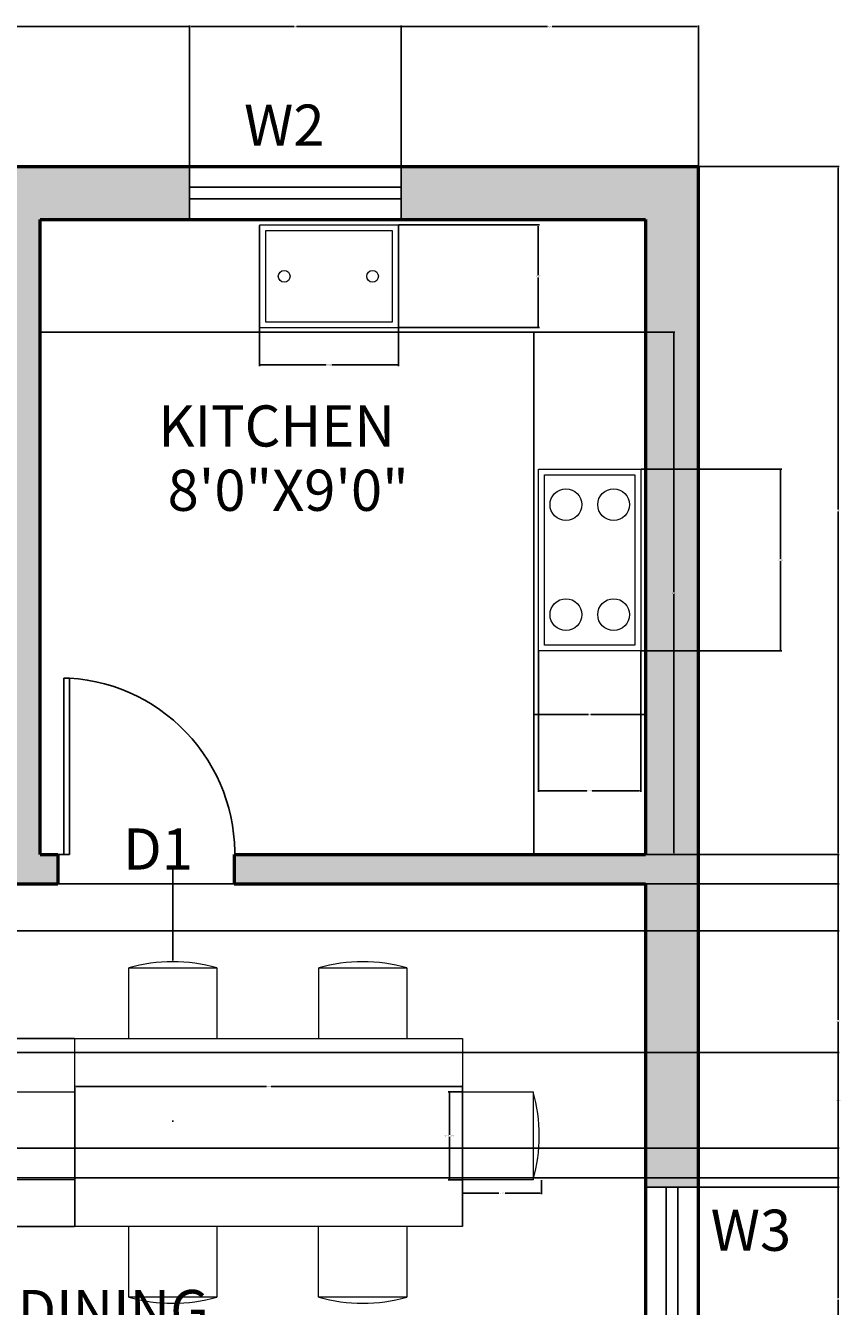
# Model space of a CAD drawing. Units: inches. Extents: x 2715 to 3027, y 1777 to 2287.
# Tile 4 of 4: x 2888 to 3027, y 2069 to 2287. Entities that reach past the tile are written whole.
import ezdxf

# ---------------------------------------------------------------- set-up
doc = ezdxf.new("R2010")
doc.units = ezdxf.units.IN
for name, color, linetype, lineweight in [('A-ANNO-DIMS', 2, 'Continuous', 18), ('A-ANNO-TEXT', 2, 'Continuous', 18), ('A-AREA-IDEN', 2, 'Continuous', 18), ('A-DOOR', 111, 'Continuous', 25), ('A-EQPM', 57, 'Continuous', 18), ('A-FLOR-CASE', 201, 'Continuous', 25), ('A-FLOR-FIXT', 201, 'Continuous', 18), ('A-FURN', 201, 'Continuous', 18), ('A-GLAZ', 40, 'Continuous', 25), ('A-WALL', 7, 'Continuous', 50), ('A-WALL-PATT', 252, 'Continuous', 13)]:
    doc.layers.add(name, color=color, linetype=linetype, lineweight=lineweight)
doc.styles.get("Standard").update_dxf_attribs({"font": 'arial.ttf'})
doc.dimstyles.get("Standard").update_dxf_attribs({"dimtxt": 0.18, "dimasz": 0.18, "dimexe": 0.18, "dimexo": 0.0625, "dimgap": 0.09, "dimtad": 0, "dimtih": 1, "dimtoh": 1, "dimdec": 4, "dimzin": 0, "dimdsep": 46, "dimtxsty": 'Standard', "dimcen": 0.09, "dimadec": 0, "dimazin": 0, "dimtfac": 1, "dimtdec": 4, "dimtofl": 0, "dimtmove": 0, "dimatfit": 3, "dimfxl": 1, "dimtolj": 1, "dimtzin": 0, "dimarcsym": 0})

# ---------------------------------------------------------------- blocks, each defined once
blk = doc.blocks.new('CHAIR-DINING')
for p, q in [((0, 0), (0, 12)), ((0, 12), (15, 12)), ((15, 12), (15, 0))]:
    blk.add_line(p, q)
blk.add_arc((7.5, -14.05), 27.1, 73.936, 106.064)
blk = doc.blocks.new('DOOR-SWING-30')
for p, q in [((29.11, 32.5), (28.11, 32.5)), ((28.11, 32.5), (28.11, 2.5)), ((29.11, 2.5), (29.11, 32.5)), ((28.11, 2.5), (29.11, 2.5)), ((30.11, 2.5), (29.11, 2.5))]:
    blk.add_line(p, q)
blk.add_arc((30, 2.56), 30, 93.6132, 184.8945)
blk = doc.blocks.new('*D11')
at = {"layer": 'A-ANNO-DIMS', "color": 0, "lineweight": -2, "transparency": 16777216}
for p, q in [((2962.73, 2105.97), (2960.36, 2105.97)), ((2960.54, 2105.79), (2960.54, 2098.66)), ((2960.54, 2091.15), (2960.54, 2098.29)), ((2962.73, 2090.97), (2960.36, 2090.97))]:
    blk.add_line(p, q, dxfattribs=at)
at = {"layer": 'A-ANNO-DIMS', "color": 0, "transparency": 16777216}
for points in [[(2960.51, 2105.79), (2960.57, 2105.79), (2960.54, 2105.97)], [(2960.51, 2091.15), (2960.57, 2091.15), (2960.54, 2090.97)]]:
    blk.add_solid(points, dxfattribs=at)
at = {"layer": 'Defpoints', "color": 0, "transparency": 16777216}
for p in [(2962.79, 2105.97), (2960.54, 2090.97), (2962.79, 2090.97)]:
    blk.add_point(p, dxfattribs=at)
at = {"layer": 'A-ANNO-DIMS', "color": 0, "transparency": 16777216, "insert": (2960.54, 2098.47), "char_height": 0.18, "attachment_point": 5}
blk.add_mtext('\\A1;CHAIR 15 TYP.', dxfattribs=at)
blk = doc.blocks.new('*D12')
at = {"layer": 'A-ANNO-DIMS', "color": 0, "lineweight": -2, "transparency": 16777216}
for p, q in [((2962.79, 2090.91), (2962.79, 2088.54)), ((2976.2, 2090.91), (2976.2, 2088.54)), ((2962.97, 2088.72), (2968.98, 2088.72)), ((2976.02, 2088.72), (2970.02, 2088.72))]:
    blk.add_line(p, q, dxfattribs=at)
at = {"layer": 'A-ANNO-DIMS', "color": 0, "transparency": 16777216}
for points in [[(2962.97, 2088.75), (2962.97, 2088.69), (2962.79, 2088.72)], [(2976.02, 2088.75), (2976.02, 2088.69), (2976.2, 2088.72)]]:
    blk.add_solid(points, dxfattribs=at)
at = {"layer": 'Defpoints', "color": 0, "transparency": 16777216}
for p in [(2962.79, 2090.97), (2976.2, 2090.97), (2976.2, 2088.72)]:
    blk.add_point(p, dxfattribs=at)
at = {"layer": 'A-ANNO-DIMS', "color": 0, "transparency": 16777216, "insert": (2969.5, 2088.72), "char_height": 0.18, "attachment_point": 5}
blk.add_mtext('\\A1;13 TYP.', dxfattribs=at)
blk = doc.blocks.new('*D30')
at = {"layer": 'A-ANNO-DIMS', "color": 0, "lineweight": -2, "transparency": 16777216}
for p, q in [((3002.98, 2089.72), (3026.9, 2089.72)), ((3026.72, 2089.54), (3026.72, 2070.9)), ((3026.72, 2051.9), (3026.72, 2070.54)), ((3002.98, 2051.72), (3026.9, 2051.72))]:
    blk.add_line(p, q, dxfattribs=at)
at = {"layer": 'A-ANNO-DIMS', "color": 0, "transparency": 16777216}
for points in [[(3026.69, 2089.54), (3026.75, 2089.54), (3026.72, 2089.72)], [(3026.69, 2051.9), (3026.75, 2051.9), (3026.72, 2051.72)]]:
    blk.add_solid(points, dxfattribs=at)
at = {"layer": 'Defpoints', "color": 0, "transparency": 16777216}
for p in [(3002.92, 2089.72), (3026.72, 2089.72), (3002.92, 2051.72)]:
    blk.add_point(p, dxfattribs=at)
at = {"layer": 'A-ANNO-DIMS', "color": 0, "transparency": 16777216, "insert": (3026.72, 2070.72), "char_height": 0.18, "attachment_point": 5}
blk.add_mtext('\\A1;38', dxfattribs=at)
blk = doc.blocks.new('*D31')
at = {"layer": 'A-ANNO-DIMS', "color": 0, "lineweight": -2, "transparency": 16777216}
for p, q in [((2993.98, 2146.34), (3026.9, 2146.34)), ((3026.72, 2146.16), (3026.72, 2118.21)), ((3026.72, 2089.9), (3026.72, 2117.85)), ((3002.98, 2089.72), (3026.9, 2089.72))]:
    blk.add_line(p, q, dxfattribs=at)
at = {"layer": 'A-ANNO-DIMS', "color": 0, "transparency": 16777216}
for points in [[(3026.69, 2146.16), (3026.75, 2146.16), (3026.72, 2146.34)], [(3026.69, 2089.9), (3026.75, 2089.9), (3026.72, 2089.72)]]:
    blk.add_solid(points, dxfattribs=at)
at = {"layer": 'Defpoints', "color": 0, "transparency": 16777216}
for p in [(2993.92, 2146.34), (3026.72, 2146.34), (3002.92, 2089.72)]:
    blk.add_point(p, dxfattribs=at)
at = {"layer": 'A-ANNO-DIMS', "color": 0, "transparency": 16777216, "insert": (3026.72, 2118.03), "char_height": 0.18, "attachment_point": 5}
blk.add_mtext('\\A1;56.62', dxfattribs=at)
blk = doc.blocks.new('*D32')
at = {"layer": 'A-ANNO-DIMS', "color": 0, "lineweight": -2, "transparency": 16777216}
for p, q in [((3002.98, 2263.34), (3026.9, 2263.34)), ((3026.72, 2263.16), (3026.72, 2205.02)), ((3026.72, 2146.52), (3026.72, 2204.66)), ((2993.98, 2146.34), (3026.9, 2146.34))]:
    blk.add_line(p, q, dxfattribs=at)
at = {"layer": 'A-ANNO-DIMS', "color": 0, "transparency": 16777216}
for points in [[(3026.69, 2263.16), (3026.75, 2263.16), (3026.72, 2263.34)], [(3026.69, 2146.52), (3026.75, 2146.52), (3026.72, 2146.34)]]:
    blk.add_solid(points, dxfattribs=at)
at = {"layer": 'Defpoints', "color": 0, "transparency": 16777216}
for p in [(3002.92, 2263.34), (3026.72, 2263.34), (2993.92, 2146.34)]:
    blk.add_point(p, dxfattribs=at)
at = {"layer": 'A-ANNO-DIMS', "color": 0, "transparency": 16777216, "insert": (3026.72, 2204.84), "char_height": 0.18, "attachment_point": 5}
blk.add_mtext('\\A1;117', dxfattribs=at)
blk = doc.blocks.new('*D35')
at = {"layer": 'A-ANNO-DIMS', "color": 0, "lineweight": -2, "transparency": 16777216}
for p, q in [((2823.27, 2263.4), (2823.27, 2287.33)), ((2823.45, 2287.15), (2869.41, 2287.15)), ((2916.16, 2287.15), (2870.19, 2287.15)), ((2916.34, 2263.4), (2916.34, 2287.33))]:
    blk.add_line(p, q, dxfattribs=at)
at = {"layer": 'A-ANNO-DIMS', "color": 0, "transparency": 16777216}
for points in [[(2823.45, 2287.18), (2823.45, 2287.12), (2823.27, 2287.15)], [(2916.16, 2287.18), (2916.16, 2287.12), (2916.34, 2287.15)]]:
    blk.add_solid(points, dxfattribs=at)
at = {"layer": 'Defpoints', "color": 0, "transparency": 16777216}
for p in [(2916.34, 2287.15), (2823.27, 2263.34), (2916.34, 2263.34)]:
    blk.add_point(p, dxfattribs=at)
at = {"layer": 'A-ANNO-DIMS', "color": 0, "transparency": 16777216, "insert": (2869.8, 2287.15), "char_height": 0.18, "attachment_point": 5}
blk.add_mtext('\\A1;93.07', dxfattribs=at)
blk = doc.blocks.new('*D36')
at = {"layer": 'A-ANNO-DIMS', "color": 0, "lineweight": -2, "transparency": 16777216}
for p, q in [((2916.34, 2263.4), (2916.34, 2287.33)), ((2916.52, 2287.15), (2934.12, 2287.15)), ((2952.16, 2287.15), (2934.55, 2287.15)), ((2952.34, 2263.4), (2952.34, 2287.33))]:
    blk.add_line(p, q, dxfattribs=at)
at = {"layer": 'A-ANNO-DIMS', "color": 0, "transparency": 16777216}
for points in [[(2916.52, 2287.18), (2916.52, 2287.12), (2916.34, 2287.15)], [(2952.16, 2287.18), (2952.16, 2287.12), (2952.34, 2287.15)]]:
    blk.add_solid(points, dxfattribs=at)
at = {"layer": 'Defpoints', "color": 0, "transparency": 16777216}
for p in [(2952.34, 2287.15), (2916.34, 2263.34), (2952.34, 2263.34)]:
    blk.add_point(p, dxfattribs=at)
at = {"layer": 'A-ANNO-DIMS', "color": 0, "transparency": 16777216, "insert": (2934.34, 2287.15), "char_height": 0.18, "attachment_point": 5}
blk.add_mtext('\\A1;36', dxfattribs=at)
blk = doc.blocks.new('*D37')
at = {"layer": 'A-ANNO-DIMS', "color": 0, "lineweight": -2, "transparency": 16777216}
for p, q in [((2952.34, 2263.4), (2952.34, 2287.33)), ((2952.52, 2287.15), (2977.23, 2287.15)), ((3002.74, 2287.15), (2978.02, 2287.15)), ((3002.92, 2263.4), (3002.92, 2287.33))]:
    blk.add_line(p, q, dxfattribs=at)
at = {"layer": 'A-ANNO-DIMS', "color": 0, "transparency": 16777216}
for points in [[(2952.52, 2287.18), (2952.52, 2287.12), (2952.34, 2287.15)], [(3002.74, 2287.18), (3002.74, 2287.12), (3002.92, 2287.15)]]:
    blk.add_solid(points, dxfattribs=at)
at = {"layer": 'Defpoints', "color": 0, "transparency": 16777216}
for p in [(3002.92, 2287.15), (2952.34, 2263.34), (3002.92, 2263.34)]:
    blk.add_point(p, dxfattribs=at)
at = {"layer": 'A-ANNO-DIMS', "color": 0, "transparency": 16777216, "insert": (2977.63, 2287.15), "char_height": 0.18, "attachment_point": 5}
blk.add_mtext('\\A1;50.58', dxfattribs=at)
blk = doc.blocks.new('*D41')
at = {"layer": 'A-ANNO-DIMS', "color": 0, "lineweight": -2, "transparency": 16777216}
for p, q in [((2747.98, 2112.64), (3026.9, 2112.64)), ((3026.72, 2112.46), (3026.72, 2104.67)), ((3026.72, 2096.52), (3026.72, 2104.31)), ((2747.98, 2096.34), (3026.9, 2096.34))]:
    blk.add_line(p, q, dxfattribs=at)
at = {"layer": 'A-ANNO-DIMS', "color": 0, "transparency": 16777216}
for points in [[(3026.69, 2112.46), (3026.75, 2112.46), (3026.72, 2112.64)], [(3026.69, 2096.52), (3026.75, 2096.52), (3026.72, 2096.34)]]:
    blk.add_solid(points, dxfattribs=at)
at = {"layer": 'Defpoints', "color": 0, "transparency": 16777216}
for p in [(2747.92, 2112.64), (3026.72, 2112.64), (2747.92, 2096.34)]:
    blk.add_point(p, dxfattribs=at)
at = {"layer": 'A-ANNO-DIMS', "color": 0, "transparency": 16777216, "insert": (3026.72, 2104.49), "char_height": 0.18, "attachment_point": 5}
blk.add_mtext('\\A1;16.297', dxfattribs=at)
blk = doc.blocks.new('*D42')
at = {"layer": 'A-ANNO-DIMS', "color": 0, "lineweight": -2, "transparency": 16777216}
for p, q in [((2831.98, 2141.34), (3026.9, 2141.34)), ((3026.72, 2141.16), (3026.72, 2137.52)), ((3026.72, 2133.52), (3026.72, 2137.16)), ((2831.98, 2133.34), (3026.9, 2133.34))]:
    blk.add_line(p, q, dxfattribs=at)
at = {"layer": 'A-ANNO-DIMS', "color": 0, "transparency": 16777216}
for points in [[(3026.69, 2141.16), (3026.75, 2141.16), (3026.72, 2141.34)], [(3026.69, 2133.52), (3026.75, 2133.52), (3026.72, 2133.34)]]:
    blk.add_solid(points, dxfattribs=at)
at = {"layer": 'Defpoints', "color": 0, "transparency": 16777216}
for p in [(2831.92, 2141.34), (3026.72, 2141.34), (2831.92, 2133.34)]:
    blk.add_point(p, dxfattribs=at)
at = {"layer": 'A-ANNO-DIMS', "color": 0, "transparency": 16777216, "insert": (3026.72, 2137.34), "char_height": 0.18, "attachment_point": 5}
blk.add_mtext('\\A1;8', dxfattribs=at)
blk = doc.blocks.new('*D43')
at = {"layer": 'A-ANNO-DIMS', "color": 0, "lineweight": -2, "transparency": 16777216}
for p, q in [((2747.98, 2096.34), (3026.9, 2096.34)), ((3026.72, 2096.16), (3026.72, 2094.02)), ((3026.72, 2091.52), (3026.72, 2093.66)), ((2747.98, 2091.34), (3026.9, 2091.34))]:
    blk.add_line(p, q, dxfattribs=at)
at = {"layer": 'A-ANNO-DIMS', "color": 0, "transparency": 16777216}
for points in [[(3026.69, 2096.16), (3026.75, 2096.16), (3026.72, 2096.34)], [(3026.69, 2091.52), (3026.75, 2091.52), (3026.72, 2091.34)]]:
    blk.add_solid(points, dxfattribs=at)
at = {"layer": 'Defpoints', "color": 0, "transparency": 16777216}
for p in [(2747.92, 2096.34), (3026.72, 2096.34), (2747.92, 2091.34)]:
    blk.add_point(p, dxfattribs=at)
at = {"layer": 'A-ANNO-DIMS', "color": 0, "transparency": 16777216, "insert": (3026.72, 2093.84), "char_height": 0.18, "attachment_point": 5}
blk.add_mtext('\\A1;5', dxfattribs=at)
blk = doc.blocks.new('*D51')
at = {"layer": 'A-ANNO-DIMS', "color": 0, "lineweight": -2, "transparency": 16777216}
for p, q in [((2896.82, 2083.1), (2896.82, 2107.02)), ((2962.79, 2083.1), (2962.79, 2107.02)), ((2897, 2106.84), (2929.41, 2106.84)), ((2962.61, 2106.84), (2930.2, 2106.84))]:
    blk.add_line(p, q, dxfattribs=at)
at = {"layer": 'A-ANNO-DIMS', "color": 0, "transparency": 16777216}
for points in [[(2897, 2106.87), (2897, 2106.81), (2896.82, 2106.84)], [(2962.61, 2106.87), (2962.61, 2106.81), (2962.79, 2106.84)]]:
    blk.add_solid(points, dxfattribs=at)
at = {"layer": 'Defpoints', "color": 0, "transparency": 16777216}
for p in [(2962.79, 2106.84), (2896.82, 2083.04), (2962.79, 2083.04)]:
    blk.add_point(p, dxfattribs=at)
at = {"layer": 'A-ANNO-DIMS', "color": 0, "transparency": 16777216, "insert": (2929.81, 2106.84), "char_height": 0.18, "attachment_point": 5}
blk.add_mtext('\\A1;65.97', dxfattribs=at)
blk = doc.blocks.new('*D52')
at = {"layer": 'A-ANNO-DIMS', "color": 0, "lineweight": -2, "transparency": 16777216}
for p, q in [((2896.76, 2115.03), (2872.84, 2115.03)), ((2873.02, 2114.85), (2873.02, 2099.21)), ((2873.02, 2083.22), (2873.02, 2098.85)), ((2896.76, 2083.04), (2872.84, 2083.04))]:
    blk.add_line(p, q, dxfattribs=at)
at = {"layer": 'A-ANNO-DIMS', "color": 0, "transparency": 16777216}
for points in [[(2872.99, 2114.85), (2873.05, 2114.85), (2873.02, 2115.03)], [(2872.99, 2083.22), (2873.05, 2083.22), (2873.02, 2083.04)]]:
    blk.add_solid(points, dxfattribs=at)
at = {"layer": 'Defpoints', "color": 0, "transparency": 16777216}
for p in [(2873.02, 2115.03), (2896.82, 2115.03), (2896.82, 2083.04)]:
    blk.add_point(p, dxfattribs=at)
at = {"layer": 'A-ANNO-DIMS', "color": 0, "transparency": 16777216, "insert": (2873.02, 2099.03), "char_height": 0.18, "attachment_point": 5}
blk.add_mtext('\\A1;31.994', dxfattribs=at)
blk = doc.blocks.new('*D53')
at = {"layer": 'A-ANNO-DIMS', "color": 0, "lineweight": -2, "transparency": 16777216}
for p, q in [((2974.92, 2146.4), (2974.92, 2170.33)), ((2975.1, 2170.15), (2984.21, 2170.15)), ((2993.74, 2170.15), (2984.63, 2170.15)), ((2993.92, 2146.4), (2993.92, 2170.33))]:
    blk.add_line(p, q, dxfattribs=at)
at = {"layer": 'A-ANNO-DIMS', "color": 0, "transparency": 16777216}
for points in [[(2975.1, 2170.18), (2975.1, 2170.12), (2974.92, 2170.15)], [(2993.74, 2170.18), (2993.74, 2170.12), (2993.92, 2170.15)]]:
    blk.add_solid(points, dxfattribs=at)
at = {"layer": 'Defpoints', "color": 0, "transparency": 16777216}
for p in [(2993.92, 2170.15), (2974.92, 2146.34), (2993.92, 2146.34)]:
    blk.add_point(p, dxfattribs=at)
at = {"layer": 'A-ANNO-DIMS', "color": 0, "transparency": 16777216, "insert": (2984.42, 2170.15), "char_height": 0.18, "attachment_point": 5}
blk.add_mtext('\\A1;19', dxfattribs=at)
blk = doc.blocks.new('*D54')
at = {"layer": 'A-ANNO-DIMS', "color": 0, "lineweight": -2, "transparency": 16777216}
for p, q in [((2974.98, 2235.2), (2998.9, 2235.2)), ((2998.72, 2235.02), (2998.72, 2190.95)), ((2998.72, 2146.52), (2998.72, 2190.59)), ((2974.98, 2146.34), (2998.9, 2146.34))]:
    blk.add_line(p, q, dxfattribs=at)
at = {"layer": 'A-ANNO-DIMS', "color": 0, "transparency": 16777216}
for points in [[(2998.69, 2235.02), (2998.75, 2235.02), (2998.72, 2235.2)], [(2998.69, 2146.52), (2998.75, 2146.52), (2998.72, 2146.34)]]:
    blk.add_solid(points, dxfattribs=at)
at = {"layer": 'Defpoints', "color": 0, "transparency": 16777216}
for p in [(2974.92, 2235.2), (2974.92, 2146.34), (2998.72, 2146.34)]:
    blk.add_point(p, dxfattribs=at)
at = {"layer": 'A-ANNO-DIMS', "color": 0, "transparency": 16777216, "insert": (2998.72, 2190.77), "char_height": 0.18, "attachment_point": 5}
blk.add_mtext('\\A1;88.86', dxfattribs=at)
blk = doc.blocks.new('*D58')
at = {"layer": 'A-ANNO-DIMS', "color": 0, "lineweight": -2, "transparency": 16777216}
for p, q in [((2928.22, 2253.34), (2928.22, 2229.42)), ((2951.88, 2253.34), (2951.88, 2229.42)), ((2928.4, 2229.6), (2939.59, 2229.6)), ((2951.7, 2229.6), (2940.51, 2229.6))]:
    blk.add_line(p, q, dxfattribs=at)
at = {"layer": 'A-ANNO-DIMS', "color": 0, "transparency": 16777216}
for points in [[(2928.4, 2229.63), (2928.4, 2229.57), (2928.22, 2229.6)], [(2951.7, 2229.63), (2951.7, 2229.57), (2951.88, 2229.6)]]:
    blk.add_solid(points, dxfattribs=at)
at = {"layer": 'Defpoints', "color": 0, "transparency": 16777216}
for p in [(2928.22, 2253.41), (2951.88, 2253.41), (2928.22, 2229.6)]:
    blk.add_point(p, dxfattribs=at)
at = {"layer": 'A-ANNO-DIMS', "color": 0, "transparency": 16777216, "insert": (2940.05, 2229.6), "char_height": 0.18, "attachment_point": 5}
blk.add_mtext('\\A1;23.654', dxfattribs=at)
blk = doc.blocks.new('*D59')
at = {"layer": 'A-ANNO-DIMS', "color": 0, "lineweight": -2, "transparency": 16777216}
for p, q in [((2951.94, 2253.41), (2975.86, 2253.41)), ((2975.68, 2253.23), (2975.68, 2244.86)), ((2975.68, 2236.13), (2975.68, 2244.5)), ((2951.94, 2235.95), (2975.86, 2235.95))]:
    blk.add_line(p, q, dxfattribs=at)
at = {"layer": 'A-ANNO-DIMS', "color": 0, "transparency": 16777216}
for points in [[(2975.65, 2253.23), (2975.71, 2253.23), (2975.68, 2253.41)], [(2975.65, 2236.13), (2975.71, 2236.13), (2975.68, 2235.95)]]:
    blk.add_solid(points, dxfattribs=at)
at = {"layer": 'Defpoints', "color": 0, "transparency": 16777216}
for p in [(2951.88, 2253.41), (2951.88, 2235.95), (2975.68, 2235.95)]:
    blk.add_point(p, dxfattribs=at)
at = {"layer": 'A-ANNO-DIMS', "color": 0, "transparency": 16777216, "insert": (2975.68, 2244.68), "char_height": 0.18, "attachment_point": 5}
blk.add_mtext('\\A1;17.453', dxfattribs=at)
blk = doc.blocks.new('*D60')
at = {"layer": 'A-ANNO-DIMS', "color": 0, "lineweight": -2, "transparency": 16777216}
for p, q in [((2993.17, 2211.88), (3017.1, 2211.88)), ((3016.92, 2211.7), (3016.92, 2196.6)), ((3016.92, 2181.14), (3016.92, 2196.24)), ((2993.17, 2180.96), (3017.1, 2180.96))]:
    blk.add_line(p, q, dxfattribs=at)
at = {"layer": 'A-ANNO-DIMS', "color": 0, "transparency": 16777216}
for points in [[(3016.89, 2211.7), (3016.95, 2211.7), (3016.92, 2211.88)], [(3016.89, 2181.14), (3016.95, 2181.14), (3016.92, 2180.96)]]:
    blk.add_solid(points, dxfattribs=at)
at = {"layer": 'Defpoints', "color": 0, "transparency": 16777216}
for p in [(2993.11, 2211.88), (2993.11, 2180.96), (3016.92, 2180.96)]:
    blk.add_point(p, dxfattribs=at)
at = {"layer": 'A-ANNO-DIMS', "color": 0, "transparency": 16777216, "insert": (3016.92, 2196.42), "char_height": 0.18, "attachment_point": 5}
blk.add_mtext('\\A1;30.924', dxfattribs=at)
blk = doc.blocks.new('*D61')
at = {"layer": 'A-ANNO-DIMS', "color": 0, "lineweight": -2, "transparency": 16777216}
for p, q in [((2975.72, 2180.89), (2975.72, 2156.97)), ((2993.11, 2180.89), (2993.11, 2156.97)), ((2975.9, 2157.15), (2983.96, 2157.15)), ((2992.93, 2157.15), (2984.87, 2157.15))]:
    blk.add_line(p, q, dxfattribs=at)
at = {"layer": 'A-ANNO-DIMS', "color": 0, "transparency": 16777216}
for points in [[(2975.9, 2157.18), (2975.9, 2157.12), (2975.72, 2157.15)], [(2992.93, 2157.18), (2992.93, 2157.12), (2993.11, 2157.15)]]:
    blk.add_solid(points, dxfattribs=at)
at = {"layer": 'Defpoints', "color": 0, "transparency": 16777216}
for p in [(2975.72, 2180.96), (2993.11, 2180.96), (2975.72, 2157.15)]:
    blk.add_point(p, dxfattribs=at)
at = {"layer": 'A-ANNO-DIMS', "color": 0, "transparency": 16777216, "insert": (2984.41, 2157.15), "char_height": 0.18, "attachment_point": 5}
blk.add_mtext('\\A1;17.394', dxfattribs=at)
blk = doc.blocks.new('*D78')
at = {"layer": 'A-ANNO-DIMS', "color": 0, "lineweight": -2, "transparency": 16777216}
for p, q in [((2913.64, 2144.35), (2913.46, 2144.35)), ((2913.46, 2144.35), (2913.46, 2128.27)), ((2913.37, 2100.98), (2913.55, 2100.98)), ((2913.46, 2100.89), (2913.46, 2101.07))]:
    blk.add_line(p, q, dxfattribs=at)
at = {"layer": 'A-ANNO-DIMS', "color": 0, "transparency": 16777216}
blk.add_solid([(2913.43, 2128.27), (2913.49, 2128.27), (2913.46, 2128.09)], dxfattribs=at)
at = {"layer": 'Defpoints', "color": 0, "transparency": 16777216}
for p in [(2913.46, 2128.09), (2913.46, 2100.98)]:
    blk.add_point(p, dxfattribs=at)
at = {"layer": 'A-ANNO-DIMS', "color": 0, "transparency": 16777216, "insert": (2914.39, 2144.35), "char_height": 0.18, "attachment_point": 5}
blk.add_mtext('\\A1;6X R27.104', dxfattribs=at)

msp = doc.modelspace()

# ---------------------------------------------------------------- hatches: boundary and pattern name
at = {"layer": 'A-WALL-PATT'}
h = msp.add_hatch(color=256, dxfattribs=at)
h.dxf.hatch_style = 1
h.paths.add_polyline_path([(2916.336, 2263.3404), (2823.2662, 2263.3404), (2823.2662, 2254.3404), (2885.9159, 2254.3404), (2885.9159, 2205.8675), (2885.9159, 2146.3404), (2882.9159, 2146.3404), (2882.9159, 2141.3404), (2893.9159, 2141.3404), (2893.9159, 2146.3404), (2890.9159, 2146.3404), (2890.9159, 2254.3404), (2916.336, 2254.3404)])
h = msp.add_hatch(color=256, dxfattribs=at)
h.dxf.hatch_style = 1
h.paths.add_polyline_path([(3002.9159, 2263.3404), (2952.336, 2263.3404), (2952.336, 2254.3404), (2993.9159, 2254.3404), (2993.9159, 2146.3404), (2924.0253, 2146.3404, -0.02086232), (2923.9159, 2143.8404), (2923.9159, 2141.3404), (2993.9159, 2141.3404), (2993.9159, 2089.722), (3002.9159, 2089.722)])

# ---------------------------------------------------------------- linework, layer by layer
at = {"layer": 'A-EQPM'}
for points in [[(2975.7156, 2211.8806), (2993.1101, 2211.8806), (2993.1101, 2180.9569), (2975.7156, 2180.9569)], [(2976.7156, 2210.8806), (2992.1101, 2210.8806), (2992.1101, 2181.9569), (2976.7156, 2181.9569)]]:
    msp.add_lwpolyline(points, close=True, dxfattribs=at)
for centre in [(2980.3732, 2205.8372), (2988.4873, 2205.8372), (2980.3732, 2187.1335), (2988.4873, 2187.1335)]:
    msp.add_circle(centre, 2.7024, dxfattribs=at)
at = {"layer": 'A-FLOR-CASE'}
for p, q in [((2890.9159, 2235.204), (2974.9159, 2235.204)), ((2974.9159, 2235.204), (2974.9159, 2146.3404))]:
    msp.add_line(p, q, dxfattribs=at)
at = {"layer": 'A-FLOR-FIXT'}
for points in [[(2951.8772, 2253.407), (2928.2231, 2253.407), (2928.2231, 2235.9536), (2951.8772, 2235.9536)], [(2950.8772, 2252.407), (2929.2231, 2252.407), (2929.2231, 2236.9536), (2950.8772, 2236.9536)]]:
    msp.add_lwpolyline(points, close=True, dxfattribs=at)
for centre in [(2932.4294, 2244.6803), (2947.473, 2244.6803)]:
    msp.add_circle(centre, 1, dxfattribs=at)
at = {"layer": 'A-FURN'}
msp.add_lwpolyline([(2896.8202, 2115.0295), (2962.7913, 2115.0295), (2962.7913, 2083.0359), (2896.8202, 2083.0359)], close=True, dxfattribs=at)
at = {"layer": 'A-GLAZ'}
for p, q in [((2916.336, 2263.3404), (2916.336, 2254.3404)), ((2952.336, 2263.3404), (2952.336, 2254.3404)), ((2916.336, 2259.8404), (2952.336, 2259.8404)), ((2916.336, 2257.8404), (2952.336, 2257.8404)), ((2993.9159, 2089.722), (3002.9159, 2089.722)), ((2997.4159, 2089.722), (2997.4159, 2051.722)), ((2999.4159, 2089.722), (2999.4159, 2051.722))]:
    msp.add_line(p, q, dxfattribs=at)
at = {"layer": 'A-WALL'}
for p, q in [((2890.9159, 2146.3404), (2890.9159, 2254.3404)), ((2890.9159, 2254.3404), (2993.9159, 2254.3404)), ((2993.9159, 2254.3404), (2993.9159, 2146.3404)), ((2890.9159, 2146.3404), (2893.9159, 2146.3404)), ((2890.9159, 2146.3404), (2893.9159, 2146.3404)), ((2893.9159, 2146.3404), (2893.9159, 2141.3404)), ((2923.9159, 2146.3404), (2923.9159, 2141.3404)), ((2923.9159, 2146.3404), (2993.9159, 2146.3404)), ((2882.9159, 2141.3404), (2893.9159, 2141.3404)), ((2923.9159, 2141.3404), (2993.9159, 2141.3404)), ((2993.9159, 2141.3404), (2993.9159, 1864.3404))]:
    msp.add_line(p, q, dxfattribs=at)
msp.add_lwpolyline([(2738.9159, 1921.3404), (2738.9159, 2263.3404), (3002.9159, 2263.3404), (3002.9159, 1855.3404), (2903.9159, 1855.3404)], dxfattribs=at)

# ---------------------------------------------------------------- block references
at = {"layer": 'A-DOOR', "extrusion": (0, 0, -1), "zscale": -1}
msp.add_blockref('DOOR-SWING-30', (-2924.0239, 2143.84), dxfattribs=at)
at = {"layer": 'A-FURN'}
for p in [(2905.962, 2115.029), (2938.2962, 2115.029)]:
    msp.add_blockref('CHAIR-DINING', p, dxfattribs=at)
for p, rotation in [((2896.8207, 2090.9735), 90), ((2962.7909, 2105.9734), 270), ((2920.9619, 2083.0364), 180), ((2953.2961, 2083.0364), 180)]:
    msp.add_blockref('CHAIR-DINING', p, dxfattribs=dict(at, rotation=rotation))

# ---------------------------------------------------------------- texts
at = {"layer": 'A-ANNO-TEXT'}
for tag, p in [('W2', (2925.6016, 2266.896)), ('D1', (2905.0207, 2143.7479)), ('W3', (3005.0203, 2078.9025))]:
    msp.add_attdef(tag, p, '', height=7, dxfattribs=at)
at = {"layer": 'A-AREA-IDEN'}
for tag, p in [('KITCHEN', (2911.0049, 2215.7231)), ('8\'0"X9\'0"', (2912.5865, 2204.7829)), ('LIVING/DINING', (2853.5433, 2065.2489))]:
    msp.add_attdef(tag, p, '', height=7, dxfattribs=at)

# ---------------------------------------------------------------- dimensions: what is measured, and where the dimension line sits
at = {"layer": 'A-ANNO-DIMS'}
for base, p1, p2, override, picture, middle in [((2916.336, 2287.1454), (2823.2662, 2263.3404), (2916.336, 2263.3404), {"dimdec": 2, "dimlfac": 1, "dimrnd": 0, "dimzin": 0, "dimdsep": 46, "dimlunit": 2}, '*D35', (2869.8011, 2287.1454)), ((2952.336, 2287.1454), (2916.336, 2263.3404), (2952.336, 2263.3404), {"dimdec": 0, "dimlfac": 1, "dimrnd": 0, "dimzin": 0, "dimdsep": 46, "dimlunit": 2}, '*D36', (2934.336, 2287.1454)), ((3002.9159, 2287.1454), (2952.336, 2263.3404), (3002.9159, 2263.3404), {"dimdec": 2, "dimlfac": 1, "dimrnd": 0, "dimzin": 0, "dimdsep": 46, "dimlunit": 2}, '*D37', (2977.626, 2287.1454)), ((2993.9159, 2170.1454), (2974.9159, 2146.3404), (2993.9159, 2146.3404), {"dimdec": 0, "dimlfac": 1, "dimrnd": 0, "dimzin": 0, "dimdsep": 46, "dimlunit": 2}, '*D53', (2984.4159, 2170.1454)), ((2962.7913, 2106.8409), (2896.8202, 2083.0359), (2962.7913, 2083.0359), {"dimdec": 2, "dimlfac": 1, "dimrnd": 0, "dimzin": 0, "dimdsep": 46, "dimlunit": 2}, '*D51', (2929.8058, 2106.8409))]:
    dim = msp.add_linear_dim(base=base, p1=p1, p2=p2, dimstyle='Standard', override=override, dxfattribs=at)
    dim.commit()
    dim.dimension.update_dxf_attribs({"geometry": picture, "text_midpoint": middle})
for base, p1, p2, angle, override, picture, middle in [((3026.7209, 2263.3404), (2993.9159, 2146.3404), (3002.9159, 2263.3404), 90, {"dimdec": 0, "dimlfac": 1, "dimrnd": 0, "dimzin": 0, "dimdsep": 46, "dimlunit": 2}, '*D32', (3026.7209, 2204.8404)), ((2928.2231, 2229.602), (2951.8772, 2253.407), (2928.2231, 2253.407), 180, {"dimdec": 3, "dimlfac": 1, "dimrnd": 0, "dimzin": 0, "dimdsep": 46, "dimlunit": 2}, '*D58', (2940.0501, 2229.602)), ((2975.6822, 2235.9536), (2951.8772, 2253.407), (2951.8772, 2235.9536), 270, {"dimdec": 3, "dimlfac": 1, "dimrnd": 0, "dimzin": 0, "dimdsep": 46, "dimlunit": 2}, '*D59', (2975.6822, 2244.6803)), ((2998.7209, 2146.3404), (2974.9159, 2235.204), (2974.9159, 2146.3404), 270, {"dimdec": 2, "dimlfac": 1, "dimrnd": 0, "dimzin": 0, "dimdsep": 46, "dimlunit": 2}, '*D54', (2998.7209, 2190.7722)), ((3016.9151, 2180.9569), (2993.1101, 2211.8806), (2993.1101, 2180.9569), 270, {"dimdec": 3, "dimlfac": 1, "dimrnd": 0, "dimzin": 0, "dimdsep": 46, "dimlunit": 2}, '*D60', (3016.9151, 2196.4187)), ((2975.71564, 2157.15188), (2993.11007, 2180.95688), (2975.71564, 2180.95688), 180, {"dimdec": 3, "dimlfac": 1, "dimrnd": 0, "dimzin": 0, "dimdsep": 46, "dimlunit": 2}, '*D61', (2984.41285, 2157.15188)), ((3026.7209, 2146.3404), (3002.9159, 2089.722), (2993.9159, 2146.3404), 90, {"dimdec": 2, "dimlfac": 1, "dimrnd": 0, "dimzin": 0, "dimdsep": 46, "dimlunit": 2}, '*D31', (3026.7209, 2118.0312)), ((3026.7209, 2141.3404), (2831.9159, 2133.3404), (2831.9159, 2141.3404), 90, {"dimdec": 0, "dimlfac": 1, "dimrnd": 0, "dimzin": 0, "dimdsep": 46, "dimlunit": 2}, '*D42', (3026.7209, 2137.3404)), ((2873.0152, 2115.0295), (2896.8202, 2083.0359), (2896.8202, 2115.0295), 90, {"dimdec": 3, "dimlfac": 1, "dimrnd": 0, "dimzin": 0, "dimdsep": 46, "dimlunit": 2}, '*D52', (2873.0152, 2099.0327)), ((3026.7209, 2112.6374), (2747.9159, 2096.3404), (2747.9159, 2112.6374), 90, {"dimdec": 3, "dimlfac": 1, "dimrnd": 0, "dimzin": 0, "dimdsep": 46, "dimlunit": 2}, '*D41', (3026.7209, 2104.4889)), ((3026.7209, 2096.3404), (2747.9159, 2091.3404), (2747.9159, 2096.3404), 90, {"dimdec": 0, "dimlfac": 1, "dimrnd": 0, "dimzin": 0, "dimdsep": 46, "dimlunit": 2}, '*D43', (3026.7209, 2093.8404)), ((3026.7209, 2089.722), (3002.9159, 2051.722), (3002.9159, 2089.722), 90, {"dimdec": 0, "dimlfac": 1, "dimrnd": 0, "dimzin": 0, "dimdsep": 46, "dimlunit": 2}, '*D30', (3026.7209, 2070.722))]:
    dim = msp.add_linear_dim(base=base, p1=p1, p2=p2, angle=angle, dimstyle='Standard', override=override, dxfattribs=at)
    dim.commit()
    dim.dimension.update_dxf_attribs({"geometry": picture, "text_midpoint": middle})
dim = msp.add_radius_dim(center=(2913.462, 2100.9838), mpoint=(2913.462, 2128.0878), text='6X <>', dimstyle='Standard', override={"dimdec": 3, "dimlfac": 1, "dimrnd": 0, "dimzin": 0, "dimdsep": 46, "dimlunit": 2}, dxfattribs=at)
dim.commit()
dim.dimension.update_dxf_attribs({"geometry": '*D78', "text_midpoint": (2914.3853, 2144.3502), "dimtype": 164})
dim = msp.add_linear_dim(base=(2960.5413, 2090.9734), p1=(2962.7913, 2105.9734), p2=(2962.7913, 2090.9734), angle=270, text='CHAIR <> TYP.', dimstyle='Standard', override={"dimdec": 0, "dimlfac": 1, "dimrnd": 0, "dimzin": 0, "dimdsep": 46, "dimlunit": 2}, dxfattribs=at)
dim.commit()
dim.dimension.update_dxf_attribs({"geometry": '*D11', "text_midpoint": (2960.5413, 2098.4734)})
dim = msp.add_linear_dim(base=(2976.2024, 2088.7234), p1=(2962.7913, 2090.9734), p2=(2976.2024, 2090.9734), text='<> TYP.', dimstyle='Standard', override={"dimdec": 0, "dimlfac": 1, "dimrnd": 0, "dimzin": 0, "dimdsep": 46, "dimlunit": 2}, dxfattribs=at)
dim.commit()
dim.dimension.update_dxf_attribs({"geometry": '*D12', "text_midpoint": (2969.4969, 2088.7234)})

doc.saveas('drawing.dxf')
